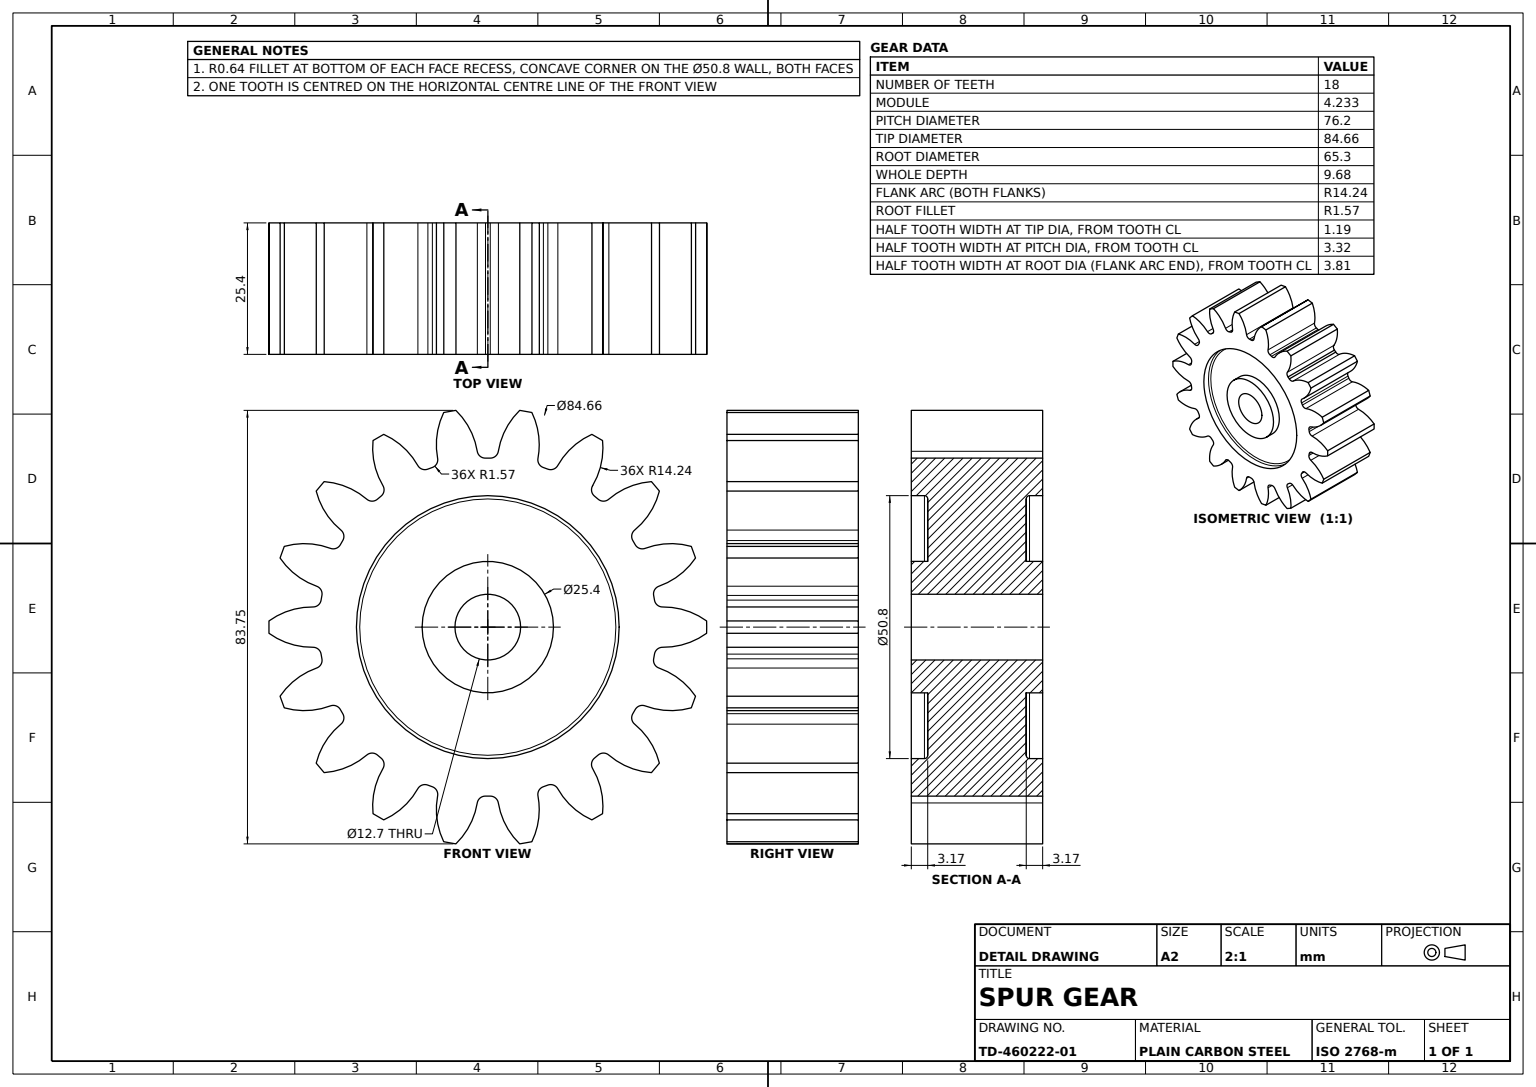
SolidWorks part; units mm, degrees
material "Plain Carbon Steel"
ref_plane "Front Plane" through (0, 0, 0) normal (0, 0, 1) x (1, 0, 0)
ref_plane "Top Plane" through (0, 0, 0) normal (0, 1, 0) x (1, 0, 0)
ref_plane "Right Plane" through (0, 0, 0) normal (1, 0, 0) x (0, 0, -1)
sketch "Gear Profile 18T Sketch" plane through (0, 0, 0) normal (0, 0, 1) x (1, 0, 0)
  line L0 (0, 72.8907) -> (0, -75.9533) construction
  line L1 (-118.981, 0) -> (116.8534, 0) construction
  circle A7 centre (0, 0) radius 6.35
  circle A8 centre (0, 0) radius 12.7
  circle A9 centre (0, 0) radius 25.4
  circle A10 centre (0, 0) radius 38.1 construction
  arc A11 (-42.3123, 1.1938) -> (-42.3123, -1.1938) centre (0, 0) ccw
  arc A12 (-32.0725, 6.1228) -> (-32.2324, 5.2159) centre (0, 0) ccw
  arc A13 (-33.8053, 3.8928) -> (-42.3123, 1.1938) centre (-33.9704, -10.3429) ccw
  arc A14 (-33.8053, 3.8928) -> (-32.2324, 5.2159) centre (-33.787, 5.4675) ccw
  arc A15 (-33.8053, -3.8928) -> (-42.3123, -1.1938) centre (-33.9704, 10.3429) cw
  arc A16 (-33.8053, -3.8928) -> (-32.2324, -5.2159) centre (-33.787, -5.4675) cw
  arc A17 (6.1718, -41.8767) -> (8.5231, -41.4621) centre (0, 0) ccw
  arc A18 (-30.4351, 15.2201) -> (-39.3522, 15.5935) centre (-35.4592, 1.8994) ccw
  arc A19 (-39.3522, 15.5935) -> (-40.1688, 13.3498) centre (0, 0) ccw
  arc A20 (-33.098, 7.9041) -> (-40.1688, 13.3498) centre (-28.3843, 21.3377) cw
  arc A21 (-33.098, 7.9041) -> (-32.0725, 6.1228) centre (-33.6194, 6.4181) cw
  arc A22 (-30.4351, 15.2201) -> (-28.5046, 15.9255) centre (-29.8794, 16.6936) ccw
  arc A23 (-23.3941, 24.7116) -> (-31.6457, 28.1123) centre (-32.6711, 13.9127) ccw
  arc A24 (-31.6457, 28.1123) -> (-33.1804, 26.2833) centre (0, 0) ccw
  arc A25 (-28.3986, 18.7476) -> (-33.1804, 26.2833) centre (-19.3746, 29.7589) cw
  arc A26 (-28.3986, 18.7476) -> (-28.0442, 16.723) centre (-29.3967, 17.5295) cw
  arc A27 (-23.3941, 24.7116) -> (-21.3387, 24.7142) centre (-22.3679, 25.9062) ccw
  arc A28 (-13.5314, 31.2226) -> (-20.1223, 37.2404) centre (-25.9424, 24.2478) ccw
  arc A29 (-20.1223, 37.2404) -> (-22.19, 36.0466) centre (0, 0) ccw
  arc A30 (-20.2739, 27.3298) -> (-22.19, 36.0466) centre (-8.028, 34.5907) cw
  arc A31 (-20.2739, 27.3298) -> (-20.6333, 25.3061) centre (-21.6285, 26.5267) cw
  arc A32 (-13.5314, 31.2226) -> (-11.5991, 30.522) centre (-12.1585, 31.9941) ccw
  arc A33 (-2.0366, 33.9676) -> (-6.1718, 41.8767) centre (-16.0847, 31.6583) ccw
  arc A34 (-6.1718, 41.8767) -> (-8.5231, 41.4621) centre (0, 0) ccw
  arc A35 (-9.7039, 32.6157) -> (-8.5231, 41.4621) centre (4.2869, 35.2504) cw
  arc A36 (-9.7039, 32.6157) -> (-10.7338, 30.837) centre (-11.2515, 32.3243) cw
  arc A37 (-2.0366, 33.9676) -> (-0.4604, 32.6485) centre (-0.4826, 34.2231) ccw
  arc A38 (9.7039, 32.6157) -> (8.5231, 41.4621) centre (-4.2869, 35.2504) ccw
  arc A39 (8.5231, 41.4621) -> (6.1718, 41.8767) centre (0, 0) ccw
  arc A40 (2.0366, 33.9676) -> (6.1718, 41.8767) centre (16.0847, 31.6583) cw
  arc A41 (2.0366, 33.9676) -> (0.4604, 32.6485) centre (0.4826, 34.2231) cw
  arc A42 (9.7039, 32.6157) -> (10.7338, 30.837) centre (11.2515, 32.3243) ccw
  arc A43 (20.2739, 27.3298) -> (22.19, 36.0466) centre (8.028, 34.5907) ccw
  arc A44 (22.19, 36.0466) -> (20.1223, 37.2404) centre (0, 0) ccw
  arc A45 (13.5314, 31.2226) -> (20.1223, 37.2404) centre (25.9424, 24.2478) cw
  arc A46 (13.5314, 31.2226) -> (11.5991, 30.522) centre (12.1585, 31.9941) cw
  arc A47 (20.2739, 27.3298) -> (20.6333, 25.3061) centre (21.6285, 26.5267) ccw
  arc A48 (28.3986, 18.7476) -> (33.1804, 26.2833) centre (19.3746, 29.7589) ccw
  arc A49 (33.1804, 26.2833) -> (31.6457, 28.1123) centre (0, 0) ccw
  arc A50 (23.3941, 24.7116) -> (31.6457, 28.1123) centre (32.6711, 13.9127) cw
  arc A51 (23.3941, 24.7116) -> (21.3387, 24.7142) centre (22.3679, 25.9062) cw
  arc A52 (28.3986, 18.7476) -> (28.0442, 16.723) centre (29.3967, 17.5295) ccw
  arc A53 (33.098, 7.9041) -> (40.1688, 13.3498) centre (28.3843, 21.3377) ccw
  arc A54 (40.1688, 13.3498) -> (39.3522, 15.5935) centre (0, 0) ccw
  arc A55 (30.4351, 15.2201) -> (39.3522, 15.5935) centre (35.4592, 1.8994) cw
  arc A56 (30.4351, 15.2201) -> (28.5046, 15.9255) centre (29.8794, 16.6936) cw
  arc A57 (33.098, 7.9041) -> (32.0725, 6.1228) centre (33.6194, 6.4181) ccw
  arc A58 (33.8053, -3.8928) -> (42.3123, -1.1938) centre (33.9704, 10.3429) ccw
  arc A59 (42.3123, -1.1938) -> (42.3123, 1.1938) centre (0, 0) ccw
  arc A60 (33.8053, 3.8928) -> (42.3123, 1.1938) centre (33.9704, -10.3429) cw
  arc A61 (33.8053, 3.8928) -> (32.2324, 5.2159) centre (33.787, 5.4675) cw
  arc A62 (33.8053, -3.8928) -> (32.2324, -5.2159) centre (33.787, -5.4675) ccw
  arc A63 (30.4351, -15.2201) -> (39.3522, -15.5935) centre (35.4592, -1.8994) ccw
  arc A64 (39.3522, -15.5935) -> (40.1688, -13.3498) centre (0, 0) ccw
  arc A65 (33.098, -7.9041) -> (40.1688, -13.3498) centre (28.3843, -21.3377) cw
  arc A66 (33.098, -7.9041) -> (32.0725, -6.1228) centre (33.6194, -6.4181) cw
  arc A67 (30.4351, -15.2201) -> (28.5046, -15.9255) centre (29.8794, -16.6936) ccw
  arc A68 (23.3941, -24.7116) -> (31.6457, -28.1123) centre (32.6711, -13.9127) ccw
  arc A69 (31.6457, -28.1123) -> (33.1804, -26.2833) centre (0, 0) ccw
  arc A70 (28.3986, -18.7476) -> (33.1804, -26.2833) centre (19.3746, -29.7589) cw
  arc A71 (28.3986, -18.7476) -> (28.0442, -16.723) centre (29.3967, -17.5295) cw
  arc A72 (23.3941, -24.7116) -> (21.3387, -24.7142) centre (22.3679, -25.9062) ccw
  arc A73 (13.5314, -31.2226) -> (20.1223, -37.2404) centre (25.9424, -24.2478) ccw
  arc A74 (20.1223, -37.2404) -> (22.19, -36.0466) centre (0, 0) ccw
  arc A75 (20.2739, -27.3298) -> (22.19, -36.0466) centre (8.028, -34.5907) cw
  arc A76 (20.2739, -27.3298) -> (20.6333, -25.3061) centre (21.6285, -26.5267) cw
  arc A77 (13.5314, -31.2226) -> (11.5991, -30.522) centre (12.1585, -31.9941) ccw
  arc A78 (2.0366, -33.9676) -> (6.1718, -41.8767) centre (16.0847, -31.6583) ccw
  arc A79 (6.1718, -41.8767) -> (8.5231, -41.4621) centre (0, 0) ccw
  arc A80 (9.7039, -32.6157) -> (8.5231, -41.4621) centre (-4.2869, -35.2504) cw
  arc A81 (9.7039, -32.6157) -> (10.7338, -30.837) centre (11.2515, -32.3243) cw
  arc A82 (2.0366, -33.9676) -> (0.4604, -32.6485) centre (0.4826, -34.2231) ccw
  arc A83 (-9.7039, -32.6157) -> (-8.5231, -41.4621) centre (4.2869, -35.2504) ccw
  arc A84 (-8.5231, -41.4621) -> (-6.1718, -41.8767) centre (0, 0) ccw
  arc A85 (-2.0366, -33.9676) -> (-6.1718, -41.8767) centre (-16.0847, -31.6583) cw
  arc A86 (-2.0366, -33.9676) -> (-0.4604, -32.6485) centre (-0.4826, -34.2231) cw
  arc A87 (-9.7039, -32.6157) -> (-10.7338, -30.837) centre (-11.2515, -32.3243) ccw
  arc A88 (-20.2739, -27.3298) -> (-22.19, -36.0466) centre (-8.028, -34.5907) ccw
  arc A89 (-22.19, -36.0466) -> (-20.1223, -37.2404) centre (0, 0) ccw
  arc A90 (-13.5314, -31.2226) -> (-20.1223, -37.2404) centre (-25.9424, -24.2478) cw
  arc A91 (-13.5314, -31.2226) -> (-11.5991, -30.522) centre (-12.1585, -31.9941) cw
  arc A92 (-20.2739, -27.3298) -> (-20.6333, -25.3061) centre (-21.6285, -26.5267) ccw
  arc A93 (-28.3986, -18.7476) -> (-33.1804, -26.2833) centre (-19.3746, -29.7589) ccw
  arc A94 (-33.1804, -26.2833) -> (-31.6457, -28.1123) centre (0, 0) ccw
  arc A95 (-23.3941, -24.7116) -> (-31.6457, -28.1123) centre (-32.6711, -13.9127) cw
  arc A96 (-23.3941, -24.7116) -> (-21.3387, -24.7142) centre (-22.3679, -25.9062) cw
  arc A97 (-28.3986, -18.7476) -> (-28.0442, -16.723) centre (-29.3967, -17.5295) ccw
  arc A98 (-33.098, -7.9041) -> (-40.1688, -13.3498) centre (-28.3843, -21.3377) ccw
  arc A99 (-40.1688, -13.3498) -> (-39.3522, -15.5935) centre (0, 0) ccw
  arc A100 (-30.4351, -15.2201) -> (-39.3522, -15.5935) centre (-35.4592, -1.8994) cw
  arc A101 (-30.4351, -15.2201) -> (-28.5046, -15.9255) centre (-29.8794, -16.6936) cw
  arc A102 (-33.098, -7.9041) -> (-32.0725, -6.1228) centre (-33.6194, -6.4181) ccw
  arc A103 (8.5231, 41.4621) -> (6.1718, 41.8767) centre (0, 0) ccw
  arc A104 (22.19, 36.0466) -> (20.1223, 37.2404) centre (0, 0) ccw
  arc A105 (33.1804, 26.2833) -> (31.6457, 28.1123) centre (0, 0) ccw
  arc A106 (40.1688, 13.3498) -> (39.3522, 15.5935) centre (0, 0) ccw
  arc A107 (42.3123, -1.1938) -> (42.3123, 1.1938) centre (0, 0) ccw
  arc A108 (39.3522, -15.5935) -> (40.1688, -13.3498) centre (0, 0) ccw
  arc A109 (31.6457, -28.1123) -> (33.1804, -26.2833) centre (0, 0) ccw
  arc A110 (20.1223, -37.2404) -> (22.19, -36.0466) centre (0, 0) ccw
  arc A111 (-28.0442, 16.723) -> (-28.5046, 15.9255) centre (0, 0) ccw
  arc A112 (-20.6333, 25.3061) -> (-21.3387, 24.7142) centre (0, 0) ccw
  arc A113 (-10.7338, 30.837) -> (-11.5991, 30.522) centre (0, 0) ccw
  arc A114 (0.4604, 32.6485) -> (-0.4604, 32.6485) centre (0, 0) ccw
  arc A115 (11.5991, 30.522) -> (10.7338, 30.837) centre (0, 0) ccw
  arc A116 (21.3387, 24.7142) -> (20.6333, 25.3061) centre (0, 0) ccw
  arc A117 (28.5046, 15.9255) -> (28.0442, 16.723) centre (0, 0) ccw
  arc A118 (32.2324, 5.2159) -> (32.0725, 6.1228) centre (0, 0) ccw
  arc A119 (32.0725, -6.1228) -> (32.2324, -5.2159) centre (0, 0) ccw
  arc A120 (28.0442, -16.723) -> (28.5046, -15.9255) centre (0, 0) ccw
  arc A121 (20.6333, -25.3061) -> (21.3387, -24.7142) centre (0, 0) ccw
  arc A122 (10.7338, -30.837) -> (11.5991, -30.522) centre (0, 0) ccw
  arc A123 (-0.4604, -32.6485) -> (0.4604, -32.6485) centre (0, 0) ccw
  arc A124 (-11.5991, -30.522) -> (-10.7338, -30.837) centre (0, 0) ccw
  arc A125 (-21.3387, -24.7142) -> (-20.6333, -25.3061) centre (0, 0) ccw
  arc A126 (-28.5046, -15.9255) -> (-28.0442, -16.723) centre (0, 0) ccw
  arc A127 (-32.2324, -5.2159) -> (-32.0725, -6.1228) centre (0, 0) ccw
  spline S0 degree 1 poles (-20.6333, 25.3061) (-21.3387, 24.7142) knots 0 0 1 1
  point P11 (-32.4287, 3.81)
  point P12 (-37.9546, 3.3249)
  point P13 (-42.3123, 1.1938)
  point P199 (0, 0)
  dimension "D1" = 12.7
  dimension "D2" = 25.4
  dimension "D3" = 50.8
  dimension "D4" = 76.2
  dimension "D5" = 84.6582
  dimension "D6" = 9.6774
  dimension "D7" = 3.81
  dimension "D8" = 3.3249
  dimension "D9" = 1.1938
  dimension "D10" = 1.5748
  dimension "D11" = 18
extrude "Gear Body 18T" add sketch "Gear Profile 18T Sketch" along normal mid plane 25.4 contours A31 S0 A27 A23 A24 A25 A26 A111 A22 A18 A19 A20 A21 A12 A14 A13 A11 A15 A16 A127 A102 A98 A99 A100 A101 A126 A97 A93 A94 A95 A96 A125 A92 A88 A89 A90 A91 A124 A87 A83 A84 A85 A86 A123 A82 A78 A17 A80 A81 A122 A77 | A9 A8 | A8 A7
sketch "Face Recess Sketch" plane through (0, 0, -12.7) normal (0, 0, -1) x (-1, 0, 0)
  circle A0 centre (0, 0) radius 25.4
  circle A1 centre (0, 0) radius 12.7
  dimension "D1" = 25.4
  dimension "D2" = 50.8
extrude "Face Recess 0.25in Deep" cut sketch "Face Recess Sketch" against normal mid plane 6.35 contours A0 A1
fillet "Recess Fillet R0.025in" radius 0.635 1 edges at (-25.4, 0, -9.525)
mirror "Face Recess Mirror" about plane through (0, 0, 0) normal (0, 0, 1) of "Recess Fillet R0.025in", "Face Recess 0.25in Deep"
